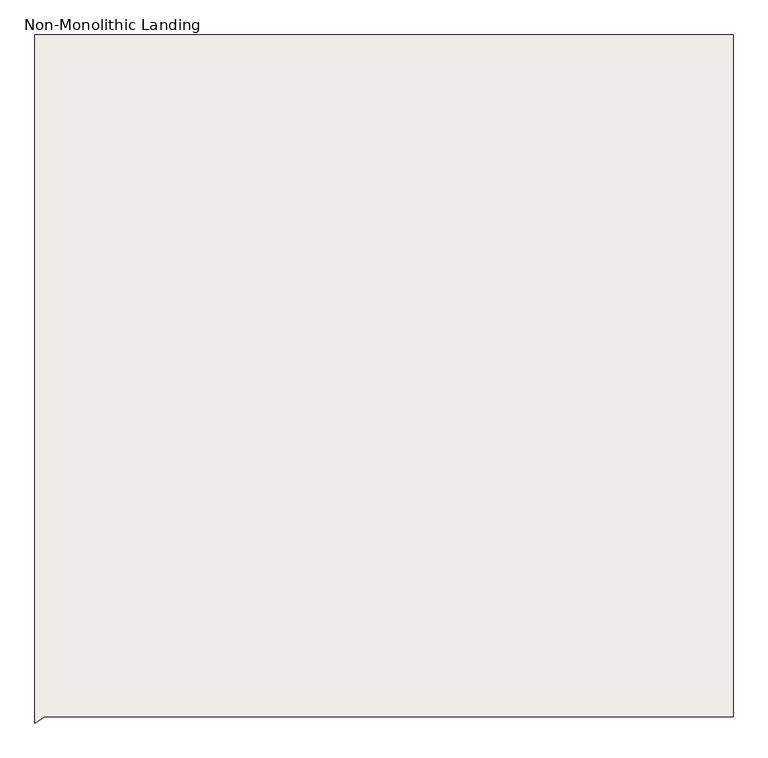
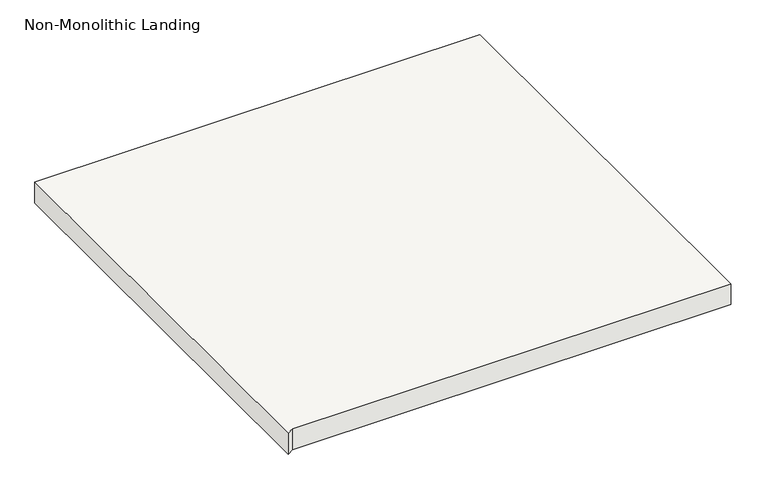
"""IFC4 building model written with IfcOpenShell, lengths in millimetres: slab geometry, Non-Monolithic Landing."""

from ifc_helpers import new_model, si_unit, frame, origin, place, context, project, spatial, polyline, outline, extrude, source, transform, mapped, element, save


def non_monolithic_landing_7cab632c(model_context):
    return source(origin(), model_context, "Body", "SweptSolid", [
        extrude(outline(polyline([(-10492.1794909, -1507.9618509), (-9477.5794909, -1507.9618509), (-9477.5794909, -2498.5618509), (-10477.6052721, -2498.5618509), (-10492.1794909, -2507.9876321), (-10492.1794909, -1507.9618509)])), frame((0.0, 0.0, 7668.6117647), z_axis=(0.0, 0.0, 1.0), x_axis=(1.0, 0.0, 0.0)), (0.0, 0.0, 1.0), 50.0),
    ])


if __name__ == "__main__":
    model = new_model("IFC4")
    model_context = context("Model", 3, world=origin())
    ifc_project = project(units=[si_unit("LENGTHUNIT", "METRE", prefix="MILLI")], contexts=[model_context])
    site = spatial("IfcSite", under=ifc_project)
    building = spatial("IfcBuilding", under=site)
    placement = place(None, origin())
    non_monolithic_landing_shape = non_monolithic_landing_7cab632c(model_context)
    element("IfcSlab", 1, ObjectType="Non-Monolithic Landing", at=placement, inside=building, context=model_context, shape_type="MappedRepresentation", body=[
        mapped(non_monolithic_landing_shape, transform((0.0, 0.0, 0.0), x_axis=(1.0, 0.0, 0.0), y_axis=(0.0, 1.0, 0.0), z_axis=(0.0, 0.0, 1.0))),
    ])
    save(model, "model.ifc")
